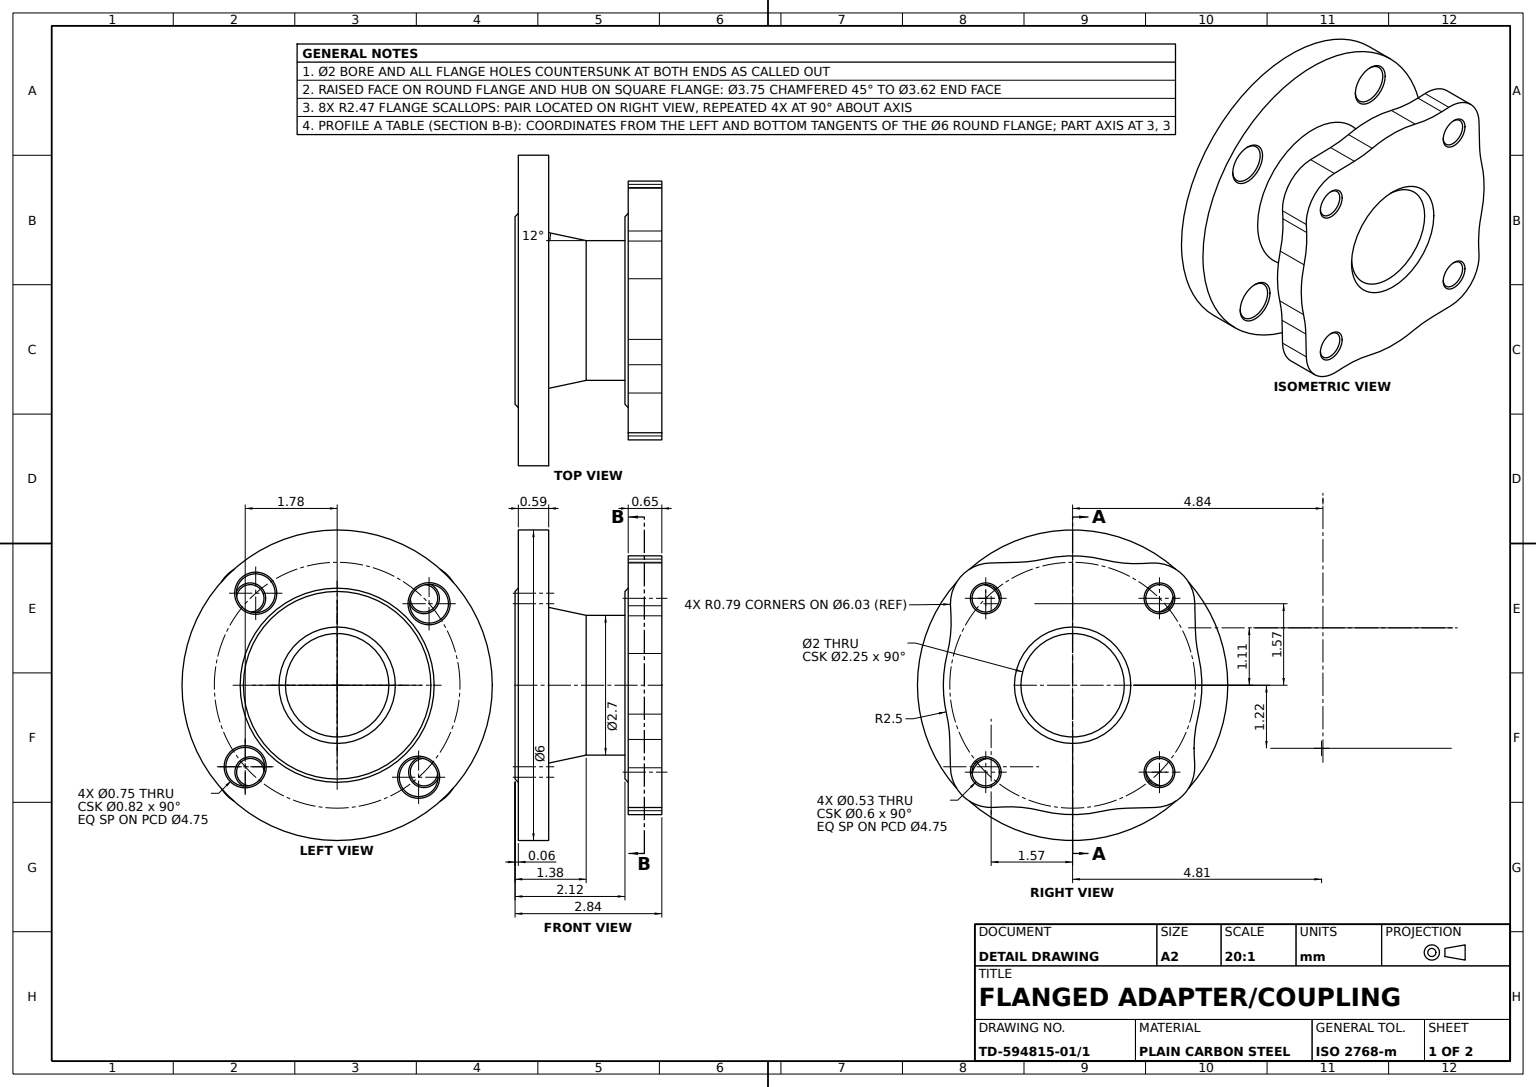
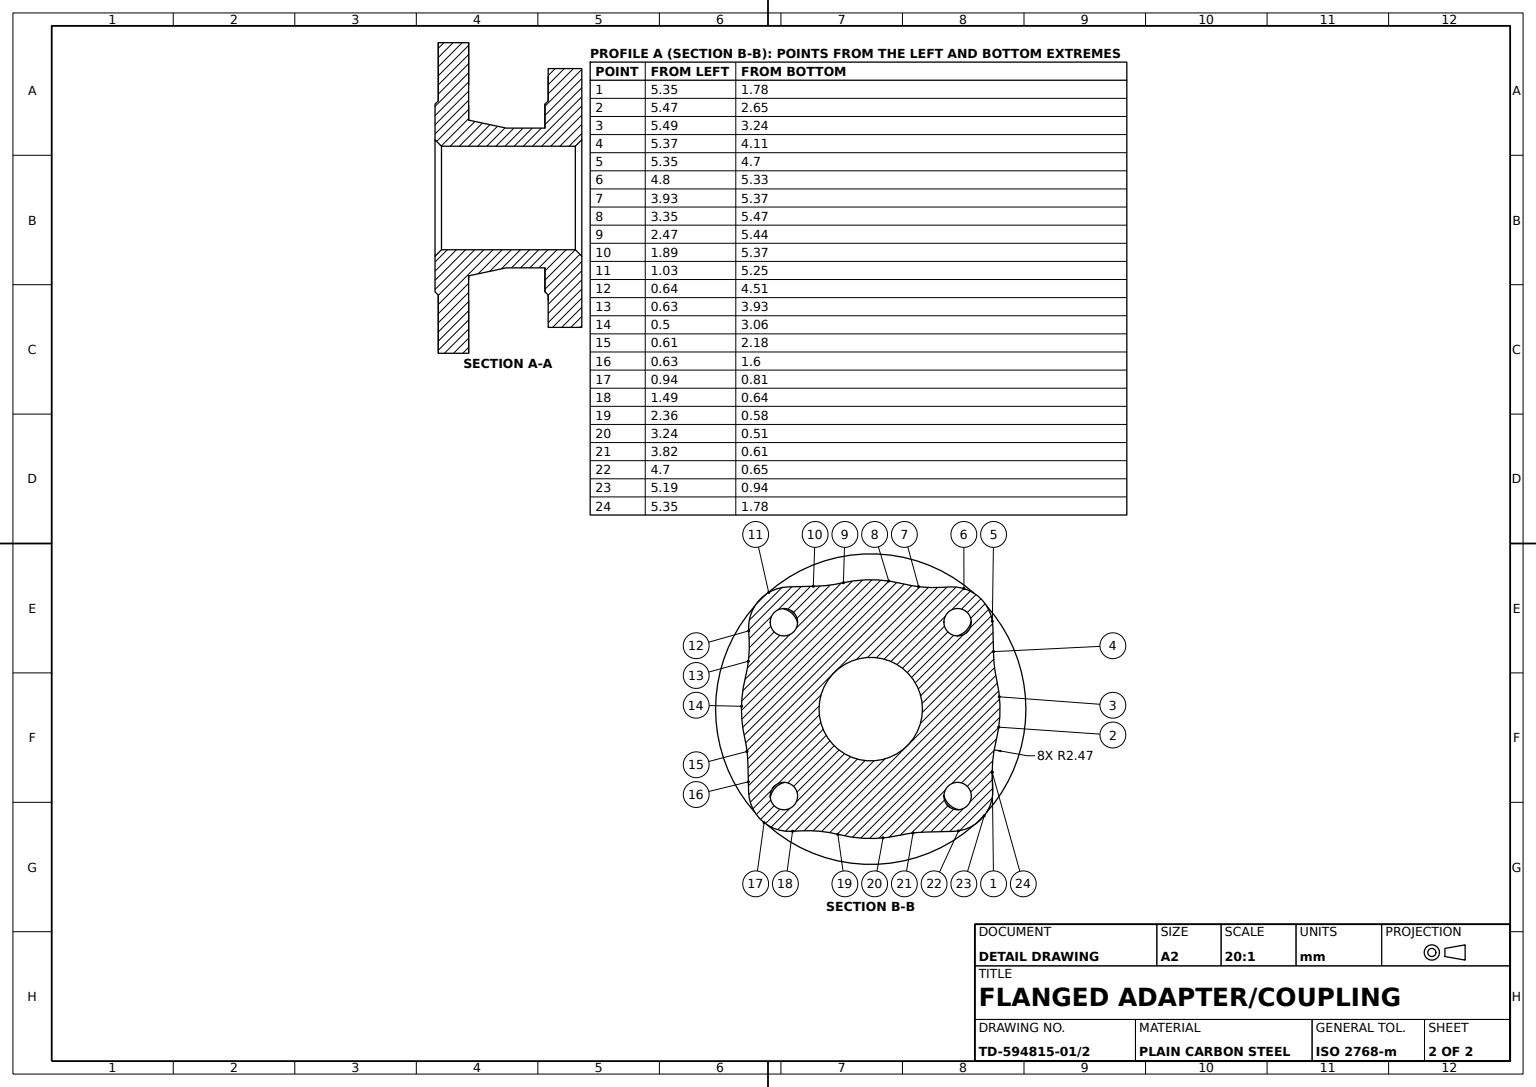
from build123d import *

# Parameters (mm, degrees)
SQUARE_FLANGE_SKETCH_R           = 1
SQUARE_FLANGE_SKETCH_R_2         = 0.265
SQUARE_OUTLET_FLANGE_DEPTH       = 0.65
ROUND_FLANGE_HOLES_SKETCH_R      = 0.375
ROUND_FLANGE_HOLES_4X_0_75_DEPTH = 0.65
ROUND_FLANGE_HOLE_CHAMFERS_SIZE  = 0.0325
SQUARE_FLANGE_CHAMFERS_SIZE      = 0.0325
HOUSING_EDGE_CHAMFERS_SIZE       = 0.125


with BuildPart() as part:
    # Housing Profile Sketch → Housing Body Revolve (revolve)
    with BuildSketch(Plane.XY, mode=Mode.PRIVATE) as housing_body_revolve_sk:
        Polygon((0, 1), (0, 1.8125), (0.063, 1.8755), (0.063, 3), (0.65, 3), (0.65, 1.504103507), (1.375, 1.35), (2.125, 1.35), (2.125, 1.812), (2.188, 1.875), (2.188, 1), align=None)
    revolve(housing_body_revolve_sk.sketch.rotate(Axis((0, 0, 0), (1, 0, 0)), 90), axis=Axis((0, 0, 0), (1, 0, 0)))

    # Square Flange Sketch → Square Outlet Flange (add)
    with BuildSketch(Plane(origin=(2.188, 0, 0), x_dir=(0, 0, -1), z_dir=(1, 0, 0))):
        with BuildLine():
            Line((-1.594555277, 2.361757009), (-1.047699115, 2.375349419))
            ThreePointArc((-1.047699115, 2.375349419), (-0.801459389, 2.393837984), (-0.558303573, 2.436862146))
            ThreePointArc((-0.558303573, 2.436862146), (0.0283118, 2.499839683), (0.613350393, 2.423592642))
            ThreePointArc((0.613350393, 2.423592642), (0.974691231, 2.360294751), (1.341424141, 2.351306033))
            Line((1.341424141, 2.351306033), (1.535705916, 2.361018432))
            ThreePointArc((1.535705916, 2.361018432), (2.110295851, 2.15191191), (2.361757009, 1.594555277))
            Line((2.361757009, 1.594555277), (2.375349419, 1.047699115))
            ThreePointArc((2.375349419, 1.047699115), (2.393837984, 0.801459389), (2.436862146, 0.558303573))
            ThreePointArc((2.436862146, 0.558303573), (2.499839683, -0.0283118), (2.423592642, -0.613350393))
            ThreePointArc((2.423592642, -0.613350393), (2.360294751, -0.974691231), (2.351306033, -1.341424141))
            Line((2.351306033, -1.341424141), (2.361018432, -1.535705916))
            ThreePointArc((2.361018432, -1.535705916), (2.15191191, -2.110295851), (1.594555277, -2.361757009))
            Line((1.594555277, -2.361757009), (1.047699115, -2.375349419))
            ThreePointArc((1.047699115, -2.375349419), (0.801459389, -2.393837984), (0.558303573, -2.436862146))
            ThreePointArc((0.558303573, -2.436862146), (-0.0283118, -2.499839683), (-0.613350393, -2.423592642))
            ThreePointArc((-0.613350393, -2.423592642), (-0.974691231, -2.360294751), (-1.341424141, -2.351306033))
            Line((-1.341424141, -2.351306033), (-1.535705916, -2.361018432))
            ThreePointArc((-1.535705916, -2.361018432), (-2.110295851, -2.15191191), (-2.361757009, -1.594555277))
            Line((-2.361757009, -1.594555277), (-2.375349419, -1.047699115))
            ThreePointArc((-2.375349419, -1.047699115), (-2.393837984, -0.801459389), (-2.436862146, -0.558303573))
            ThreePointArc((-2.436862146, -0.558303573), (-2.499839683, 0.0283118), (-2.423592642, 0.613350393))
            ThreePointArc((-2.423592642, 0.613350393), (-2.360294751, 0.974691231), (-2.351306033, 1.341424141))
            Line((-2.351306033, 1.341424141), (-2.361018432, 1.535705916))
            ThreePointArc((-2.361018432, 1.535705916), (-2.15191191, 2.110295851), (-1.594555277, 2.361757009))
        make_face()
        with Locations(Location((0, 0, 0), (0, 0, 180))):
            Circle(SQUARE_FLANGE_SKETCH_R, mode=Mode.SUBTRACT)
        with Locations((-1.679378605, 1.679378605)):
            Circle(SQUARE_FLANGE_SKETCH_R_2, mode=Mode.SUBTRACT)
        with Locations((1.679378605, 1.679378605)):
            Circle(SQUARE_FLANGE_SKETCH_R_2, mode=Mode.SUBTRACT)
        with Locations((1.679378605, -1.679378605)):
            Circle(SQUARE_FLANGE_SKETCH_R_2, mode=Mode.SUBTRACT)
        with Locations((-1.679378605, -1.679378605)):
            Circle(SQUARE_FLANGE_SKETCH_R_2, mode=Mode.SUBTRACT)
    extrude(amount=SQUARE_OUTLET_FLANGE_DEPTH)

    # Round Flange Holes Sketch → Round Flange Holes 4xØ0.75 (cut)
    with BuildSketch(Plane.ZY.offset(-0.063)):
        with Locations((-1.575, 1.777638883)):
            Circle(ROUND_FLANGE_HOLES_SKETCH_R)
        with Locations((1.777638883, 1.575)):
            Circle(ROUND_FLANGE_HOLES_SKETCH_R)
        with Locations((1.575, -1.777638883)):
            Circle(ROUND_FLANGE_HOLES_SKETCH_R)
        with Locations((-1.777638883, -1.575)):
            Circle(ROUND_FLANGE_HOLES_SKETCH_R)
    extrude(amount=-ROUND_FLANGE_HOLES_4X_0_75_DEPTH, mode=Mode.SUBTRACT)

    # Round Flange Hole Chamfers
    round_flange_hole_chamfers_edges = [part.edges().sort_by_distance(p)[0] for p in [
        (0.65, -1.777638883, 1.2),
        (0.063, -1.777638883, 1.2),
        (0.65, 1.575, 1.402638883),
        (0.063, 1.575, 1.402638883),
        (0.65, 1.777638883, -1.95),
        (0.063, 1.777638883, -1.95),
        (0.65, -1.575, -2.152638883),
        (0.063, -1.575, -2.152638883),
    ]]
    chamfer(round_flange_hole_chamfers_edges, length=ROUND_FLANGE_HOLE_CHAMFERS_SIZE)

    # Square Flange Chamfers
    square_flange_chamfers_edges = [part.edges().sort_by_distance(p)[0] for p in [
        (2.188, 1.679378605, 1.944378605),
        (2.188, 1.679378605, -1.414378605),
        (2.188, -1.679378605, -1.414378605),
        (2.188, -1.679378605, 1.944378605),
        (2.838, 1.679378605, 1.944378605),
        (2.838, 1.679378605, -1.414378605),
        (2.838, -1.679378605, -1.414378605),
        (2.838, -1.679378605, 1.944378605),
    ]]
    chamfer(square_flange_chamfers_edges, length=SQUARE_FLANGE_CHAMFERS_SIZE)

    # Housing Edge Chamfers
    housing_edge_chamfers_edges = [part.edges().sort_by_distance(p)[0] for p in [
        (0, 0, -1),
        (2.838, 0, -1),
    ]]
    chamfer(housing_edge_chamfers_edges, length=HOUSING_EDGE_CHAMFERS_SIZE)


solid = part.part
